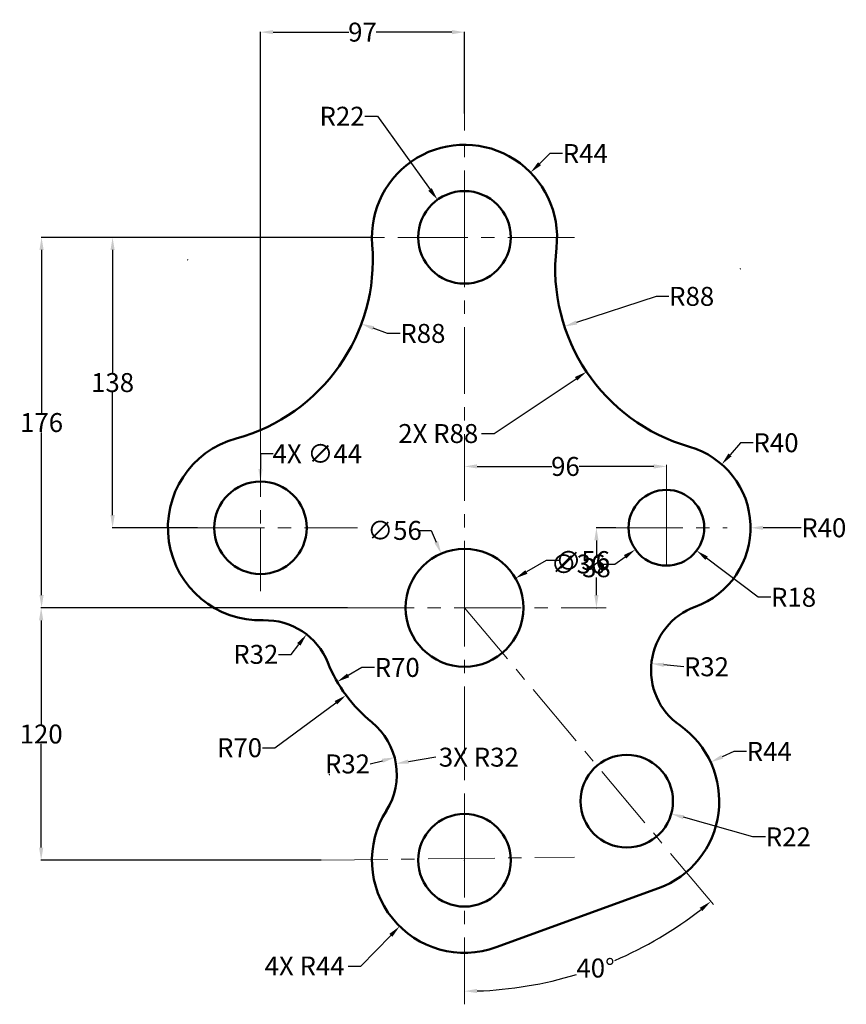
# Model space of a CAD drawing. Units: inches. Extents: x 84 to 477, y 98 to 566.
import ezdxf

# ---------------------------------------------------------------- set-up
doc = ezdxf.new("R2010")
doc.units = ezdxf.units.IN
doc.header["$MEASUREMENT"] = 0
doc.linetypes.add('CENTER', pattern=[50.8, 31.75, -6.35, 6.35, -6.35])
for name, color, linetype, lineweight in [('M-CNTR', 4, 'CENTER', 18), ('M-DIMS', 2, 'Continuous', 25), ('M-OUTL', 7, 'Continuous', 50)]:
    doc.layers.add(name, color=color, linetype=linetype, lineweight=lineweight)
doc.styles.get("Standard").update_dxf_attribs({"font": 'arial.ttf'})
doc.dimstyles.get("Standard").update_dxf_attribs({"dimtxt": 9, "dimasz": 6, "dimexe": 0.18, "dimexo": 0.0625, "dimgap": 0.09, "dimtad": 0, "dimtih": 1, "dimtoh": 1, "dimdec": 0, "dimzin": 0, "dimdsep": 46, "dimtxsty": 'Standard', "dimcen": 0.09, "dimclrd": 1, "dimclre": 1, "dimadec": 0, "dimazin": 0, "dimtfac": 1, "dimtdec": 0, "dimtofl": 0, "dimtmove": 0, "dimatfit": 3, "dimfxl": 1, "dimtolj": 1, "dimtzin": 0, "dimarcsym": 0})

# ---------------------------------------------------------------- blocks, each defined once
blk = doc.blocks.new('*D1')
at = {"layer": 'Defpoints', "color": 0, "transparency": 16777216}
for p in [(327.27, 493.24), (295.86, 462.43)]:
    blk.add_point(p, dxfattribs=at)
at = {"layer": 'M-DIMS', "color": 0, "lineweight": -2, "transparency": 16777216}
for p, q in [((336.48, 502.26), (331.56, 497.44)), ((342.48, 502.26), (336.48, 502.26)), ((295.77, 462.43), (295.95, 462.43)), ((295.86, 462.34), (295.86, 462.52))]:
    blk.add_line(p, q, dxfattribs=at)
at = {"layer": 'M-DIMS', "color": 0, "transparency": 16777216}
blk.add_solid([(330.86, 498.15), (332.26, 496.72), (327.27, 493.24)], dxfattribs=at)
at = {"layer": 'M-DIMS', "color": 0, "transparency": 16777216, "insert": (353.3, 502.26), "char_height": 9, "attachment_point": 5}
blk.add_mtext('\\A1;R44', dxfattribs=at)
blk = doc.blocks.new('*D2')
at = {"layer": 'Defpoints', "color": 0, "transparency": 16777216}
for p in [(198.86, 559.95), (295.86, 521.23), (198.86, 370.9)]:
    blk.add_point(p, dxfattribs=at)
at = {"layer": 'M-DIMS', "color": 0, "lineweight": -2, "transparency": 16777216}
for p, q in [((198.86, 370.96), (198.86, 560.13)), ((204.86, 559.95), (240.82, 559.95)), ((289.86, 559.95), (253.89, 559.95)), ((295.86, 521.29), (295.86, 560.13))]:
    blk.add_line(p, q, dxfattribs=at)
at = {"layer": 'M-DIMS', "color": 0, "transparency": 16777216}
for points in [[(204.86, 560.95), (204.86, 558.95), (198.86, 559.95)], [(289.86, 560.95), (289.86, 558.95), (295.86, 559.95)]]:
    blk.add_solid(points, dxfattribs=at)
at = {"layer": 'M-DIMS', "color": 0, "transparency": 16777216, "insert": (247.36, 559.95), "char_height": 9, "attachment_point": 5}
blk.add_mtext('\\A1;97', dxfattribs=at)
blk = doc.blocks.new('*D3')
at = {"layer": 'Defpoints', "color": 0, "transparency": 16777216}
for p in [(283.01, 480.29), (295.86, 462.43)]:
    blk.add_point(p, dxfattribs=at)
at = {"layer": 'M-DIMS', "color": 0, "lineweight": -2, "transparency": 16777216}
for p, q in [((248.45, 519.98), (254.45, 519.98)), ((254.45, 519.98), (279.5, 485.16)), ((295.77, 462.43), (295.95, 462.43)), ((295.86, 462.34), (295.86, 462.52))]:
    blk.add_line(p, q, dxfattribs=at)
at = {"layer": 'M-DIMS', "color": 0, "transparency": 16777216}
blk.add_solid([(280.31, 485.74), (278.69, 484.57), (283.01, 480.29)], dxfattribs=at)
at = {"layer": 'M-DIMS', "color": 0, "transparency": 16777216, "insert": (237.65, 519.98), "char_height": 9, "attachment_point": 5}
blk.add_mtext('\\A1;R22', dxfattribs=at)
blk = doc.blocks.new('*D4')
at = {"layer": 'Defpoints', "color": 0, "transparency": 16777216}
for p in [(427.01, 447.51), (343.39, 420.08)]:
    blk.add_point(p, dxfattribs=at)
at = {"layer": 'M-DIMS', "color": 0, "lineweight": -2, "transparency": 16777216}
for p, q in [((387.02, 434.39), (349.09, 421.95)), ((393.02, 434.39), (387.02, 434.39))]:
    blk.add_line(p, q, dxfattribs=at)
at = {"layer": 'M-DIMS', "color": 0, "transparency": 16777216}
blk.add_solid([(348.78, 422.9), (349.41, 421), (343.39, 420.08)], dxfattribs=at)
at = {"layer": 'M-DIMS', "color": 0, "transparency": 16777216, "insert": (403.87, 434.39), "char_height": 9, "attachment_point": 5}
blk.add_mtext('\\A1;R88', dxfattribs=at)
blk = doc.blocks.new('*D5')
at = {"layer": 'Defpoints', "color": 0, "transparency": 16777216}
for p in [(418.16, 354.56), (391.86, 324.43)]:
    blk.add_point(p, dxfattribs=at)
at = {"layer": 'M-DIMS', "color": 0, "lineweight": -2, "transparency": 16777216}
for p, q in [((427.14, 364.84), (422.11, 359.08)), ((433.14, 364.84), (427.14, 364.84)), ((391.77, 324.43), (391.95, 324.43)), ((391.86, 324.34), (391.86, 324.52))]:
    blk.add_line(p, q, dxfattribs=at)
at = {"layer": 'M-DIMS', "color": 0, "transparency": 16777216}
blk.add_solid([(421.36, 359.74), (422.86, 358.42), (418.16, 354.56)], dxfattribs=at)
at = {"layer": 'M-DIMS', "color": 0, "transparency": 16777216, "insert": (443.97, 364.84), "char_height": 9, "attachment_point": 5}
blk.add_mtext('\\A1;R40', dxfattribs=at)
blk = doc.blocks.new('*D6')
at = {"layer": 'Defpoints', "color": 0, "transparency": 16777216}
for p in [(295.86, 353.58), (295.86, 353.58), (391.86, 353.58)]:
    blk.add_point(p, dxfattribs=at)
at = {"layer": 'M-DIMS', "color": 0, "lineweight": -2, "transparency": 16777216}
for p, q in [((295.86, 353.65), (295.86, 353.76)), ((301.86, 353.58), (337.32, 353.58)), ((385.86, 353.58), (350.39, 353.58)), ((391.86, 353.65), (391.86, 353.76))]:
    blk.add_line(p, q, dxfattribs=at)
at = {"layer": 'M-DIMS', "color": 0, "transparency": 16777216}
for points in [[(301.86, 354.58), (301.86, 352.58), (295.86, 353.58)], [(385.86, 354.58), (385.86, 352.58), (391.86, 353.58)]]:
    blk.add_solid(points, dxfattribs=at)
at = {"layer": 'M-DIMS', "color": 0, "transparency": 16777216, "insert": (343.86, 353.58), "char_height": 9, "attachment_point": 5}
blk.add_mtext('\\A1;96', dxfattribs=at)
blk = doc.blocks.new('*D7')
at = {"layer": 'Defpoints', "color": 0, "transparency": 16777216}
for p in [(367.89, 324.43), (358.58, 286.43), (358.58, 286.43)]:
    blk.add_point(p, dxfattribs=at)
at = {"layer": 'M-DIMS', "color": 0, "lineweight": -2, "transparency": 16777216}
for p, q in [((367.83, 324.43), (358.4, 324.43)), ((358.58, 318.43), (358.58, 310.12)), ((358.58, 292.43), (358.58, 300.74)), ((358.64, 286.43), (358.76, 286.43))]:
    blk.add_line(p, q, dxfattribs=at)
at = {"layer": 'M-DIMS', "color": 0, "transparency": 16777216}
for points in [[(357.58, 318.43), (359.58, 318.43), (358.58, 324.43)], [(357.58, 292.43), (359.58, 292.43), (358.58, 286.43)]]:
    blk.add_solid(points, dxfattribs=at)
at = {"layer": 'M-DIMS', "color": 0, "transparency": 16777216, "insert": (358.58, 305.43), "char_height": 9, "attachment_point": 5}
blk.add_mtext('\\A1;38', dxfattribs=at)
blk = doc.blocks.new('*D8')
at = {"layer": 'Defpoints', "color": 0, "transparency": 16777216}
for p in [(284.8, 312.15), (306.92, 260.71)]:
    blk.add_point(p, dxfattribs=at)
at = {"layer": 'M-DIMS', "color": 0, "lineweight": -2, "transparency": 16777216}
for p, q in [((274.06, 323.18), (280.06, 323.18)), ((280.06, 323.18), (282.43, 317.66)), ((295.77, 286.43), (295.95, 286.43)), ((295.86, 286.34), (295.86, 286.52))]:
    blk.add_line(p, q, dxfattribs=at)
at = {"layer": 'M-DIMS', "color": 0, "transparency": 16777216}
blk.add_solid([(283.34, 318.06), (281.51, 317.27), (284.8, 312.15)], dxfattribs=at)
at = {"layer": 'M-DIMS', "color": 0, "transparency": 16777216, "insert": (262.63, 323.18), "char_height": 9, "attachment_point": 5}
blk.add_mtext('\\A1;∅56', dxfattribs=at)
blk = doc.blocks.new('*D9')
at = {"layer": 'Defpoints', "color": 0, "transparency": 16777216}
for p in [(391.86, 324.43), (406.21, 313.56)]:
    blk.add_point(p, dxfattribs=at)
at = {"layer": 'M-DIMS', "color": 0, "lineweight": -2, "transparency": 16777216}
for p, q in [((391.77, 324.43), (391.95, 324.43)), ((391.86, 324.34), (391.86, 324.52)), ((435.47, 291.41), (410.99, 309.94)), ((441.47, 291.41), (435.47, 291.41))]:
    blk.add_line(p, q, dxfattribs=at)
at = {"layer": 'M-DIMS', "color": 0, "transparency": 16777216}
blk.add_solid([(411.59, 310.74), (410.39, 309.14), (406.21, 313.56)], dxfattribs=at)
at = {"layer": 'M-DIMS', "color": 0, "transparency": 16777216, "insert": (452.32, 291.41), "char_height": 9, "attachment_point": 5}
blk.add_mtext('\\A1;R18', dxfattribs=at)
blk = doc.blocks.new('*D10')
at = {"layer": 'Defpoints', "color": 0, "transparency": 16777216}
for p in [(384.69, 259.88), (416.54, 256.79)]:
    blk.add_point(p, dxfattribs=at)
at = {"layer": 'M-DIMS', "color": 0, "lineweight": -2, "transparency": 16777216}
blk.add_line((400.09, 258.39), (390.66, 259.3), dxfattribs=at)
at = {"layer": 'M-DIMS', "color": 0, "transparency": 16777216}
blk.add_solid([(390.76, 260.3), (390.56, 258.31), (384.69, 259.88)], dxfattribs=at)
at = {"layer": 'M-DIMS', "color": 0, "transparency": 16777216, "insert": (410.89, 258.39), "char_height": 9, "attachment_point": 5}
blk.add_mtext('\\A1;R32', dxfattribs=at)
blk = doc.blocks.new('*D11')
at = {"layer": 'Defpoints', "color": 0, "transparency": 16777216}
for p in [(412.89, 213.06), (372.99, 194.5)]:
    blk.add_point(p, dxfattribs=at)
at = {"layer": 'M-DIMS', "color": 0, "lineweight": -2, "transparency": 16777216}
for p, q in [((423.91, 218.18), (418.33, 215.59)), ((429.91, 218.18), (423.91, 218.18)), ((372.9, 194.5), (373.08, 194.5)), ((372.99, 194.41), (372.99, 194.59))]:
    blk.add_line(p, q, dxfattribs=at)
at = {"layer": 'M-DIMS', "color": 0, "transparency": 16777216}
blk.add_solid([(417.91, 216.5), (418.75, 214.68), (412.89, 213.06)], dxfattribs=at)
at = {"layer": 'M-DIMS', "color": 0, "transparency": 16777216, "insert": (440.73, 218.18), "char_height": 9, "attachment_point": 5}
blk.add_mtext('\\A1;R44', dxfattribs=at)
blk = doc.blocks.new('*D12')
at = {"layer": 'Defpoints', "color": 0, "transparency": 16777216}
for p in [(372.99, 194.5), (394.16, 188.52)]:
    blk.add_point(p, dxfattribs=at)
at = {"layer": 'M-DIMS', "color": 0, "lineweight": -2, "transparency": 16777216}
for p, q in [((372.9, 194.5), (373.08, 194.5)), ((372.99, 194.41), (372.99, 194.59)), ((433.02, 177.54), (399.94, 186.89)), ((439.02, 177.54), (433.02, 177.54))]:
    blk.add_line(p, q, dxfattribs=at)
at = {"layer": 'M-DIMS', "color": 0, "transparency": 16777216}
blk.add_solid([(400.21, 187.85), (399.66, 185.93), (394.16, 188.52)], dxfattribs=at)
at = {"layer": 'M-DIMS', "color": 0, "transparency": 16777216, "insert": (449.82, 177.54), "char_height": 9, "attachment_point": 5}
blk.add_mtext('\\A1;R22', dxfattribs=at)
blk = doc.blocks.new('*D13')
at = {"layer": 'Defpoints', "color": 0, "transparency": 16777216}
for p in [(295.86, 286.43), (295.86, 166.43), (414.61, 144.91), (337.87, 109.15), (295.86, 98)]:
    blk.add_point(p, dxfattribs=at)
at = {"layer": 'M-DIMS', "color": 0, "lineweight": -2, "transparency": 16777216}
for start, end in [(293.0768, 308.113), (271.887, 286.9823)]:
    blk.add_arc((295.86, 286.43), 182.19, start, end, dxfattribs=at)
at = {"layer": 'M-DIMS', "color": 0, "transparency": 16777216}
for points in [[(407.68, 143.86), (408.94, 142.31), (412.96, 146.87)], [(301.87, 103.34), (301.84, 105.34), (295.86, 104.24)]]:
    blk.add_solid(points, dxfattribs=at)
at = {"layer": 'M-DIMS', "color": 0, "transparency": 16777216, "insert": (358.17, 115.23), "char_height": 9, "attachment_point": 5}
blk.add_mtext('\\A1;40°', dxfattribs=at)
blk = doc.blocks.new('*D14')
at = {"layer": 'Defpoints', "color": 0, "transparency": 16777216}
for p in [(262.64, 215.27), (231.68, 207.15)]:
    blk.add_point(p, dxfattribs=at)
at = {"layer": 'M-DIMS', "color": 0, "lineweight": -2, "transparency": 16777216}
blk.add_line((251.03, 212.22), (256.83, 213.75), dxfattribs=at)
at = {"layer": 'M-DIMS', "color": 0, "transparency": 16777216}
blk.add_solid([(256.58, 214.71), (257.09, 212.78), (262.64, 215.27)], dxfattribs=at)
at = {"layer": 'M-DIMS', "color": 0, "transparency": 16777216, "insert": (240.23, 212.22), "char_height": 9, "attachment_point": 5}
blk.add_mtext('\\A1;R32', dxfattribs=at)
blk = doc.blocks.new('*D15')
at = {"layer": 'Defpoints', "color": 0, "transparency": 16777216}
for p in [(295.86, 286.43), (235.34, 251.25)]:
    blk.add_point(p, dxfattribs=at)
at = {"layer": 'M-DIMS', "color": 0, "lineweight": -2, "transparency": 16777216}
for p, q in [((247.06, 258.07), (240.53, 254.27)), ((253.06, 258.07), (247.06, 258.07))]:
    blk.add_line(p, q, dxfattribs=at)
at = {"layer": 'M-DIMS', "color": 0, "transparency": 16777216}
blk.add_solid([(240.02, 255.13), (241.03, 253.4), (235.34, 251.25)], dxfattribs=at)
at = {"layer": 'M-DIMS', "color": 0, "transparency": 16777216, "insert": (263.89, 258.07), "char_height": 9, "attachment_point": 5}
blk.add_mtext('\\A1;R70', dxfattribs=at)
blk = doc.blocks.new('*D16')
at = {"layer": 'Defpoints', "color": 0, "transparency": 16777216}
for p in [(220.78, 273.77), (201.19, 248.47)]:
    blk.add_point(p, dxfattribs=at)
at = {"layer": 'M-DIMS', "color": 0, "lineweight": -2, "transparency": 16777216}
for p, q in [((213.43, 264.28), (217.1, 269.02)), ((207.43, 264.28), (213.43, 264.28))]:
    blk.add_line(p, q, dxfattribs=at)
at = {"layer": 'M-DIMS', "color": 0, "transparency": 16777216}
blk.add_solid([(216.31, 269.64), (217.89, 268.41), (220.78, 273.77)], dxfattribs=at)
at = {"layer": 'M-DIMS', "color": 0, "transparency": 16777216, "insert": (196.63, 264.28), "char_height": 9, "attachment_point": 5}
blk.add_mtext('\\A1;R32', dxfattribs=at)
blk = doc.blocks.new('*D17')
at = {"layer": 'Defpoints', "color": 0, "transparency": 16777216}
for p in [(164.28, 451.82), (246.84, 421.36)]:
    blk.add_point(p, dxfattribs=at)
at = {"layer": 'M-DIMS', "color": 0, "lineweight": -2, "transparency": 16777216}
for p, q in [((164.19, 451.82), (164.37, 451.82)), ((164.28, 451.73), (164.28, 451.91)), ((259.23, 416.79), (252.47, 419.28)), ((265.23, 416.79), (259.23, 416.79))]:
    blk.add_line(p, q, dxfattribs=at)
at = {"layer": 'M-DIMS', "color": 0, "transparency": 16777216}
blk.add_solid([(252.82, 420.22), (252.13, 418.35), (246.84, 421.36)], dxfattribs=at)
at = {"layer": 'M-DIMS', "color": 0, "transparency": 16777216, "insert": (276.08, 416.79), "char_height": 9, "attachment_point": 5}
blk.add_mtext('\\A1;R88', dxfattribs=at)
blk = doc.blocks.new('*D18')
at = {"layer": 'Defpoints', "color": 0, "transparency": 16777216}
for p in [(251.86, 462.43), (128.55, 324.43), (169, 324.43)]:
    blk.add_point(p, dxfattribs=at)
at = {"layer": 'M-DIMS', "color": 0, "lineweight": -2, "transparency": 16777216}
for p, q in [((251.79, 462.43), (128.37, 462.43)), ((128.55, 456.43), (128.55, 398.12)), ((128.55, 330.43), (128.55, 388.74)), ((168.94, 324.43), (128.37, 324.43))]:
    blk.add_line(p, q, dxfattribs=at)
at = {"layer": 'M-DIMS', "color": 0, "transparency": 16777216}
for points in [[(127.55, 456.43), (129.55, 456.43), (128.55, 462.43)], [(127.55, 330.43), (129.55, 330.43), (128.55, 324.43)]]:
    blk.add_solid(points, dxfattribs=at)
at = {"layer": 'M-DIMS', "color": 0, "transparency": 16777216, "insert": (128.55, 393.43), "char_height": 9, "attachment_point": 5}
blk.add_mtext('\\A1;138', dxfattribs=at)
blk = doc.blocks.new('*D19')
at = {"layer": 'Defpoints', "color": 0, "transparency": 16777216}
for p in [(94.78, 462.43), (251.86, 462.43), (240.23, 286.43)]:
    blk.add_point(p, dxfattribs=at)
at = {"layer": 'M-DIMS', "color": 0, "lineweight": -2, "transparency": 16777216}
for p, q in [((251.79, 462.43), (94.6, 462.43)), ((94.78, 456.43), (94.78, 379.11)), ((94.78, 292.43), (94.78, 369.74)), ((240.16, 286.43), (94.6, 286.43))]:
    blk.add_line(p, q, dxfattribs=at)
at = {"layer": 'M-DIMS', "color": 0, "transparency": 16777216}
for points in [[(93.78, 456.43), (95.78, 456.43), (94.78, 462.43)], [(93.78, 292.43), (95.78, 292.43), (94.78, 286.43)]]:
    blk.add_solid(points, dxfattribs=at)
at = {"layer": 'M-DIMS', "color": 0, "transparency": 16777216, "insert": (94.78, 374.43), "char_height": 9, "attachment_point": 5}
blk.add_mtext('\\A1;176', dxfattribs=at)
blk = doc.blocks.new('*D20')
at = {"layer": 'Defpoints', "color": 0, "transparency": 16777216}
for p in [(240.23, 286.43), (94.6, 166.43), (227.72, 166.43)]:
    blk.add_point(p, dxfattribs=at)
at = {"layer": 'M-DIMS', "color": 0, "lineweight": -2, "transparency": 16777216}
for p, q in [((240.16, 286.43), (94.42, 286.43)), ((94.6, 280.43), (94.6, 231.11)), ((94.6, 172.43), (94.6, 221.74)), ((227.66, 166.43), (94.42, 166.43))]:
    blk.add_line(p, q, dxfattribs=at)
at = {"layer": 'M-DIMS', "color": 0, "transparency": 16777216}
for points in [[(93.6, 280.43), (95.6, 280.43), (94.6, 286.43)], [(93.6, 172.43), (95.6, 172.43), (94.6, 166.43)]]:
    blk.add_solid(points, dxfattribs=at)
at = {"layer": 'M-DIMS', "color": 0, "transparency": 16777216, "insert": (94.6, 226.43), "char_height": 9, "attachment_point": 5}
blk.add_mtext('\\A1;120', dxfattribs=at)
blk = doc.blocks.new('HUB-BORE-D44')
blk.add_circle((22, 22), 22)
blk = doc.blocks.new('*D22')
at = {"layer": 'Defpoints', "color": 0, "transparency": 16777216}
for p in [(427.01, 447.51), (353.87, 398.57)]:
    blk.add_point(p, dxfattribs=at)
at = {"layer": 'M-DIMS', "color": 1, "lineweight": -2, "transparency": 16777216}
for p, q in [((426.92, 447.51), (427.1, 447.51)), ((427.01, 447.42), (427.01, 447.6)), ((309.99, 369.21), (348.88, 395.24)), ((303.99, 369.21), (309.99, 369.21))]:
    blk.add_line(p, q, dxfattribs=at)
at = {"layer": 'M-DIMS', "color": 1, "transparency": 16777216}
blk.add_solid([(348.33, 396.07), (349.44, 394.41), (353.87, 398.57)], dxfattribs=at)
at = {"layer": 'M-DIMS', "color": 0, "transparency": 16777216, "insert": (283.39, 369.21), "char_height": 9, "attachment_point": 5}
blk.add_mtext('\\A1;2X R88', dxfattribs=at)
blk = doc.blocks.new('*D23')
at = {"layer": 'Defpoints', "color": 0, "transparency": 16777216}
for p in [(295.86, 286.43), (239.54, 244.86)]:
    blk.add_point(p, dxfattribs=at)
at = {"layer": 'M-DIMS', "color": 1, "lineweight": -2, "transparency": 16777216}
for p, q in [((295.77, 286.43), (295.95, 286.43)), ((295.86, 286.34), (295.86, 286.52)), ((205.75, 219.92), (234.71, 241.3)), ((199.75, 219.92), (205.75, 219.92))]:
    blk.add_line(p, q, dxfattribs=at)
at = {"layer": 'M-DIMS', "color": 1, "transparency": 16777216}
blk.add_solid([(234.12, 242.1), (235.3, 240.49), (239.54, 244.86)], dxfattribs=at)
at = {"layer": 'M-DIMS', "color": 0, "transparency": 16777216, "insert": (188.92, 219.92), "char_height": 9, "attachment_point": 5}
blk.add_mtext('\\A1;R70', dxfattribs=at)
blk = doc.blocks.new('*D24')
at = {"layer": 'Defpoints', "color": 0, "transparency": 16777216}
for p in [(295.86, 166.43), (265.03, 135.03)]:
    blk.add_point(p, dxfattribs=at)
at = {"layer": 'M-DIMS', "color": 1, "lineweight": -2, "transparency": 16777216}
for p, q in [((295.77, 166.43), (295.95, 166.43)), ((295.86, 166.34), (295.86, 166.52)), ((246.54, 116.19), (260.83, 130.75)), ((240.54, 116.19), (246.54, 116.19))]:
    blk.add_line(p, q, dxfattribs=at)
at = {"layer": 'M-DIMS', "color": 1, "transparency": 16777216}
blk.add_solid([(260.11, 131.45), (261.54, 130.05), (265.03, 135.03)], dxfattribs=at)
at = {"layer": 'M-DIMS', "color": 0, "transparency": 16777216, "insert": (219.86, 116.19), "char_height": 9, "attachment_point": 5}
blk.add_mtext('\\A1;4X R44', dxfattribs=at)
blk = doc.blocks.new('*D25')
at = {"layer": 'Defpoints', "color": 0, "transparency": 16777216}
for p in [(391.86, 324.43), (431.86, 324.43)]:
    blk.add_point(p, dxfattribs=at)
at = {"layer": 'M-DIMS', "color": 1, "lineweight": -2, "transparency": 16777216}
for p, q in [((391.77, 324.43), (391.95, 324.43)), ((391.86, 324.34), (391.86, 324.52)), ((455.86, 324.43), (437.86, 324.43))]:
    blk.add_line(p, q, dxfattribs=at)
at = {"layer": 'M-DIMS', "color": 1, "transparency": 16777216}
blk.add_solid([(437.86, 325.43), (437.86, 323.43), (431.86, 324.43)], dxfattribs=at)
at = {"layer": 'M-DIMS', "color": 0, "transparency": 16777216, "insert": (466.68, 324.43), "char_height": 9, "attachment_point": 5}
blk.add_mtext('\\A1;R40', dxfattribs=at)
blk = doc.blocks.new('*D26')
at = {"layer": 'Defpoints', "color": 0, "transparency": 16777216}
for p in [(263.26, 212.32), (231.68, 207.15)]:
    blk.add_point(p, dxfattribs=at)
at = {"layer": 'M-DIMS', "color": 1, "lineweight": -2, "transparency": 16777216}
for p, q in [((282.21, 215.43), (269.18, 213.29)), ((231.59, 207.15), (231.77, 207.15)), ((231.68, 207.06), (231.68, 207.24))]:
    blk.add_line(p, q, dxfattribs=at)
at = {"layer": 'M-DIMS', "color": 1, "transparency": 16777216}
blk.add_solid([(269.02, 214.28), (269.35, 212.31), (263.26, 212.32)], dxfattribs=at)
at = {"layer": 'M-DIMS', "color": 0, "transparency": 16777216, "insert": (302.67, 215.43), "char_height": 9, "attachment_point": 5}
blk.add_mtext('\\A1;3X R32', dxfattribs=at)
blk = doc.blocks.new('*D27')
at = {"layer": 'Defpoints', "color": 0, "transparency": 16777216}
for p in [(320.1, 300.43), (271.61, 272.43)]:
    blk.add_point(p, dxfattribs=at)
at = {"layer": 'M-DIMS', "color": 1, "lineweight": -2, "transparency": 16777216}
for p, q in [((334.65, 308.83), (325.3, 303.43)), ((340.65, 308.83), (334.65, 308.83)), ((295.77, 286.43), (295.95, 286.43)), ((295.86, 286.34), (295.86, 286.52))]:
    blk.add_line(p, q, dxfattribs=at)
at = {"layer": 'M-DIMS', "color": 1, "transparency": 16777216}
blk.add_solid([(324.8, 304.3), (325.8, 302.57), (320.1, 300.43)], dxfattribs=at)
at = {"layer": 'M-DIMS', "color": 0, "transparency": 16777216, "insert": (352.08, 308.83), "char_height": 9, "attachment_point": 5}
blk.add_mtext('\\A1;∅56', dxfattribs=at)
blk = doc.blocks.new('*D28')
at = {"layer": 'Defpoints', "color": 0, "transparency": 16777216}
for p in [(198.86, 346.43), (198.86, 302.43)]:
    blk.add_point(p, dxfattribs=at)
at = {"layer": 'M-DIMS', "color": 1, "lineweight": -2, "transparency": 16777216}
for p, q in [((204.86, 359.63), (198.86, 359.63)), ((198.86, 359.63), (198.86, 352.43)), ((198.77, 324.43), (198.95, 324.43)), ((198.86, 324.34), (198.86, 324.52))]:
    blk.add_line(p, q, dxfattribs=at)
at = {"layer": 'M-DIMS', "color": 1, "transparency": 16777216}
blk.add_solid([(197.86, 352.43), (199.86, 352.43), (198.86, 346.43)], dxfattribs=at)
at = {"layer": 'M-DIMS', "color": 0, "transparency": 16777216, "insert": (225.88, 359.63), "char_height": 9, "attachment_point": 5}
blk.add_mtext('\\A1;4X ∅44', dxfattribs=at)
blk = doc.blocks.new('*D29')
at = {"layer": 'Defpoints', "color": 0, "transparency": 16777216}
for p in [(406.6, 334.76), (377.12, 314.1)]:
    blk.add_point(p, dxfattribs=at)
at = {"layer": 'M-DIMS', "color": 1, "lineweight": -2, "transparency": 16777216}
for p, q in [((391.77, 324.43), (391.95, 324.43)), ((391.86, 324.34), (391.86, 324.52)), ((367.29, 307.21), (372.2, 310.65)), ((361.29, 307.21), (367.29, 307.21))]:
    blk.add_line(p, q, dxfattribs=at)
at = {"layer": 'M-DIMS', "color": 1, "transparency": 16777216}
blk.add_solid([(371.63, 311.47), (372.78, 309.84), (377.12, 314.1)], dxfattribs=at)
at = {"layer": 'M-DIMS', "color": 0, "transparency": 16777216, "insert": (349.86, 307.21), "char_height": 9, "attachment_point": 5}
blk.add_mtext('\\A1;∅36', dxfattribs=at)

msp = doc.modelspace()

# ---------------------------------------------------------------- linework, layer by layer
at = {"layer": 'M-CNTR'}
for p, q in [((391.86, 324.43), (391.86, 354.38)), ((169, 324.43), (244.92, 324.43)), ((367.89, 324.43), (420.79, 324.43)), ((391.86, 306.43), (391.86, 324.43)), ((240.23, 286.43), (363.14, 286.43)), ((295.86, 286.43), (414.61, 144.91)), ((227.72, 166.43), (348.17, 167.96))]:
    msp.add_line(p, q, dxfattribs=at)
for points in [[(348.2, 462.43), (295.86, 462.43), (295.86, 521.23)], [(295.86, 98), (295.86, 166.43), (295.86, 286.43), (295.86, 462.43), (251.86, 462.43)], [(198.86, 370.9), (198.86, 324.43), (198.86, 294.36)]]:
    msp.add_lwpolyline(points, dxfattribs=at)
at = {"layer": 'M-OUTL'}
msp.add_line((310.91, 125.08), (388.04, 153.16), dxfattribs=at)
for centre, radius in [((391.86, 324.43), 18), ((295.86, 286.43), 28)]:
    msp.add_circle(centre, radius, dxfattribs=at)
for centre, radius, start, end in [((295.86, 462.43), 44, 353.5091, 184.6095), ((164.28, 451.82), 88, 285.1838, 4.6095), ((427.01, 447.51), 88, 173.5091, 254.0595), ((198.86, 324.43), 44, 105.1838, 271.7556), ((391.86, 324.43), 40, 290.0467, 74.0595), ((416.54, 256.79), 32, 110.0467, 235.0421), ((201.19, 248.47), 32, 21.8513, 91.7556), ((295.86, 286.43), 70, 201.8513, 231.0129), ((231.68, 207.15), 32, 327.6055, 51.0129), ((372.99, 194.5), 44, 290, 55.0421), ((295.86, 166.43), 44, 147.6055, 290)]:
    msp.add_arc(centre, radius, start, end, dxfattribs=at)

# ---------------------------------------------------------------- block references
for p in [(273.86, 440.43), (176.86, 302.43), (350.99, 172.5), (273.86, 144.43)]:
    msp.add_blockref('HUB-BORE-D44', p, dxfattribs=at)

# ---------------------------------------------------------------- dimensions: what is measured, and where the dimension line sits
at = {"layer": 'M-DIMS'}
dim = msp.add_linear_dim(base=(198.86, 559.95), p1=(295.86, 521.23), p2=(198.86, 370.9), dimstyle='Standard', override={"dimclrd": 0, "dimclre": 0, "dimclrt": 0}, dxfattribs=at)
dim.commit()
dim.dimension.update_dxf_attribs({"geometry": '*D2', "text_midpoint": (247.36, 559.95)})
for center, mpoint, override, picture, middle in [((295.86, 462.43), (283.01, 480.29), {"dimclrd": 0, "dimclre": 0, "dimclrt": 0}, '*D3', (237.65, 519.98)), ((295.86, 462.43), (327.27, 493.24), {"dimclrd": 0, "dimclre": 0, "dimclrt": 0}, '*D1', (353.3, 502.26)), ((164.28, 451.82), (246.84, 421.36), {"dimclrd": 0, "dimclre": 0, "dimclrt": 0}, '*D17', (276.08, 416.79)), ((427.01, 447.51), (343.39, 420.08), {"dimclrd": 0, "dimclre": 0, "dimclrt": 0}, '*D4', (403.87, 434.39)), ((391.86, 324.43), (418.16, 354.56), {"dimclrd": 0, "dimclre": 0, "dimclrt": 0}, '*D5', (443.97, 364.84)), ((391.86, 324.43), (431.86, 324.43), {"dimdec": 0, "dimlfac": 1, "dimrnd": 0, "dimzin": 0, "dimdsep": 46, "dimlunit": 2}, '*D25', (455.86, 324.43)), ((391.86, 324.43), (406.21, 313.56), {"dimclrd": 0, "dimclre": 0, "dimclrt": 0}, '*D9', (452.32, 291.41)), ((295.86, 286.43), (239.54, 244.86), {"dimdec": 0, "dimlfac": 1, "dimrnd": 0, "dimzin": 0, "dimdsep": 46, "dimlunit": 2}, '*D23', (188.92, 219.92)), ((295.86, 286.43), (235.34, 251.25), {"dimclrd": 0, "dimclre": 0, "dimclrt": 0}, '*D15', (263.89, 258.07)), ((201.19, 248.47), (220.78, 273.77), {"dimclrd": 0, "dimclre": 0, "dimclrt": 0}, '*D16', (196.63, 264.28)), ((416.54, 256.79), (384.69, 259.88), {"dimclrd": 0, "dimclre": 0, "dimclrt": 0}, '*D10', (400.09, 258.39)), ((372.99, 194.5), (412.89, 213.06), {"dimclrd": 0, "dimclre": 0, "dimclrt": 0}, '*D11', (440.73, 218.18)), ((231.68, 207.15), (262.64, 215.27), {"dimclrd": 0, "dimclre": 0, "dimclrt": 0}, '*D14', (251.03, 212.22)), ((372.99, 194.5), (394.16, 188.52), {"dimclrd": 0, "dimclre": 0, "dimclrt": 0}, '*D12', (449.82, 177.54))]:
    dim = msp.add_radius_dim(center=center, mpoint=mpoint, dimstyle='Standard', override=override, dxfattribs=at)
    dim.commit()
    dim.dimension.update_dxf_attribs({"geometry": picture, "text_midpoint": middle, "dimtype": 164})
for base, p1, p2, angle, picture, middle in [((94.78, 462.43), (240.23, 286.43), (251.86, 462.43), 90, '*D19', (94.78, 374.43)), ((128.55, 324.43), (251.86, 462.43), (169, 324.43), 90, '*D18', (128.55, 393.43)), ((295.86, 353.58), (391.86, 353.58), (295.86, 353.58), 180, '*D6', (343.86, 353.58)), ((358.58, 286.43), (367.89, 324.43), (358.58, 286.43), 90, '*D7', (358.58, 305.43)), ((94.6, 166.43), (240.23, 286.43), (227.72, 166.43), 90, '*D20', (94.6, 226.43))]:
    dim = msp.add_linear_dim(base=base, p1=p1, p2=p2, angle=angle, dimstyle='Standard', override={"dimclrd": 0, "dimclre": 0, "dimclrt": 0}, dxfattribs=at)
    dim.commit()
    dim.dimension.update_dxf_attribs({"geometry": picture, "text_midpoint": middle})
for center, mpoint, text, picture, middle in [((427.01, 447.51), (353.87, 398.57), '2X <>', '*D22', (283.39, 369.21)), ((231.68, 207.15), (263.26, 212.32), '3X <>', '*D26', (282.21, 215.43)), ((295.86, 166.43), (265.03, 135.03), '4X <>', '*D24', (219.86, 116.19))]:
    dim = msp.add_radius_dim(center=center, mpoint=mpoint, text=text, dimstyle='Standard', override={"dimdec": 0, "dimlfac": 1, "dimrnd": 0, "dimzin": 0, "dimdsep": 46, "dimlunit": 2}, dxfattribs=at)
    dim.commit()
    dim.dimension.update_dxf_attribs({"geometry": picture, "text_midpoint": middle, "dimtype": 164})
dim = msp.add_diameter_dim_2p(p1=(198.86, 302.43), p2=(198.86, 346.43), text='4X <>', dimstyle='Standard', override={"dimdec": 0, "dimlfac": 1, "dimrnd": 0, "dimzin": 0, "dimdsep": 46, "dimlunit": 2}, dxfattribs=at)
dim.commit()
dim.dimension.update_dxf_attribs({"geometry": '*D28', "text_midpoint": (225.88, 359.63), "dimtype": 163})
for p1, p2, override, picture, middle in [((406.6, 334.76), (377.12, 314.1), {"dimdec": 0, "dimlfac": 1, "dimrnd": 0, "dimzin": 0, "dimdsep": 46, "dimlunit": 2}, '*D29', (349.86, 307.21)), ((306.92, 260.71), (284.8, 312.15), {"dimclrd": 0, "dimclre": 0, "dimclrt": 0}, '*D8', (262.63, 323.18)), ((271.61, 272.43), (320.1, 300.43), {"dimdec": 0, "dimlfac": 1, "dimrnd": 0, "dimzin": 0, "dimdsep": 46, "dimlunit": 2}, '*D27', (352.08, 308.83))]:
    dim = msp.add_diameter_dim_2p(p1=p1, p2=p2, dimstyle='Standard', override=override, dxfattribs=at)
    dim.commit()
    dim.dimension.update_dxf_attribs({"geometry": picture, "text_midpoint": middle, "dimtype": 163})
dim = msp.add_angular_dim_2l(base=(337.87, 109.15), line1=((295.86, 286.43), (414.61, 144.91)), line2=((295.86, 98), (295.86, 166.43)), dimstyle='Standard', override={"dimclrd": 0, "dimclre": 0, "dimclrt": 0}, dxfattribs=at)
dim.commit()
dim.dimension.update_dxf_attribs({"geometry": '*D13', "text_midpoint": (358.17, 115.23)})

doc.saveas('drawing.dxf')
